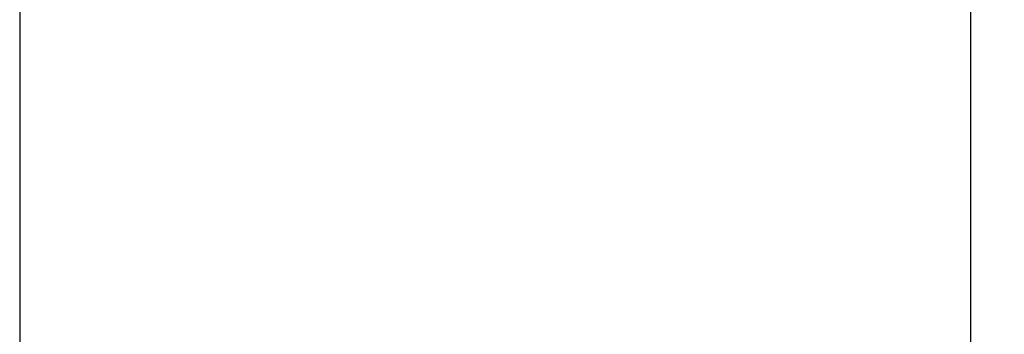
# Model space of a CAD drawing. Units: inches. Extents: x 2091 to 2899, y 967 to 2217.
# Tile 3 of 256: x 2212 to 2312, y 1033 to 1065. Entities that reach past the tile are written whole.
import ezdxf

# ---------------------------------------------------------------- set-up
doc = ezdxf.new("R2010")
doc.units = ezdxf.units.IN
doc.layers.add('A-ANNO-DIMS', color=2, linetype='Continuous', lineweight=18)
doc.styles.get("Standard").update_dxf_attribs({"font": 'arial.ttf'})
doc.dimstyles.new('ISO-25', dxfattribs={"dimtxt": 4, "dimasz": 4, "dimexe": 1.25, "dimexo": 0.625, "dimtad": 1, "dimdec": 0, "dimlunit": 3, "dimtxsty": 'Standard', "dimcen": 2.5, "dimadec": 0, "dimazin": 0, "dimtfac": 1, "dimtdec": 0, "dimtmove": 0, "dimatfit": 3, "dimfxl": 1, "dimarcsym": 0})

# ---------------------------------------------------------------- blocks, each defined once
blk = doc.blocks.new('*D71')
at = {"layer": 'A-ANNO-DIMS', "color": 0, "lineweight": -2, "transparency": 16777216}
for p, q in [((2212.144, 1351.294), (2212.144, 969.464)), ((2452.144, 1351.294), (2452.144, 969.464)), ((2216.144, 970.714), (2448.144, 970.714))]:
    blk.add_line(p, q, dxfattribs=at)
at = {"layer": 'A-ANNO-DIMS', "color": 0, "transparency": 16777216}
for points in [[(2216.144, 971.381), (2216.144, 970.048), (2212.144, 970.714)], [(2448.144, 971.381), (2448.144, 970.048), (2452.144, 970.714)]]:
    blk.add_solid(points, dxfattribs=at)
at = {"layer": 'Defpoints', "color": 0, "transparency": 16777216}
for p in [(2212.144, 1351.919), (2452.144, 1351.919), (2452.144, 970.714)]:
    blk.add_point(p, dxfattribs=at)
at = {"layer": 'A-ANNO-DIMS', "color": 0, "transparency": 16777216, "insert": (2332.144, 973.382), "char_height": 4, "attachment_point": 5}
blk.add_mtext('20\'-0"', dxfattribs=at)
blk = doc.blocks.new('*D75')
at = {"layer": 'A-ANNO-DIMS', "color": 0, "lineweight": -2, "transparency": 16777216}
for p, q in [((2212.144, 1274.794), (2212.144, 969.464)), ((2308.144, 1274.794), (2308.144, 969.464)), ((2216.144, 970.714), (2304.144, 970.714))]:
    blk.add_line(p, q, dxfattribs=at)
at = {"layer": 'A-ANNO-DIMS', "color": 0, "transparency": 16777216}
for points in [[(2216.144, 971.381), (2216.144, 970.048), (2212.144, 970.714)], [(2304.144, 971.381), (2304.144, 970.048), (2308.144, 970.714)]]:
    blk.add_solid(points, dxfattribs=at)
at = {"layer": 'Defpoints', "color": 0, "transparency": 16777216}
for p in [(2212.144, 1275.419), (2308.144, 1275.419), (2308.144, 970.714)]:
    blk.add_point(p, dxfattribs=at)
at = {"layer": 'A-ANNO-DIMS', "color": 0, "transparency": 16777216, "insert": (2260.144, 973.382), "char_height": 4, "attachment_point": 5}
blk.add_mtext('8\'-0"', dxfattribs=at)

msp = doc.modelspace()

# ---------------------------------------------------------------- dimensions: what is measured, and where the dimension line sits
at = {"layer": 'A-ANNO-DIMS'}
for base, p1, p2, picture, middle in [((2452.144, 970.714), (2212.144, 1351.919), (2452.144, 1351.919), '*D71', (2332.144, 973.382)), ((2308.144, 970.714), (2212.144, 1275.419), (2308.144, 1275.419), '*D75', (2260.144, 973.382))]:
    dim = msp.add_linear_dim(base=base, p1=p1, p2=p2, dimstyle='ISO-25', override={"dimdec": 1, "dimlfac": 1, "dimrnd": 0, "dimzin": 1, "dimdsep": 46, "dimlunit": 4, "dimfrac": 2}, dxfattribs=at)
    dim.commit()
    dim.dimension.update_dxf_attribs({"geometry": picture, "text_midpoint": middle})

doc.saveas('drawing.dxf')
